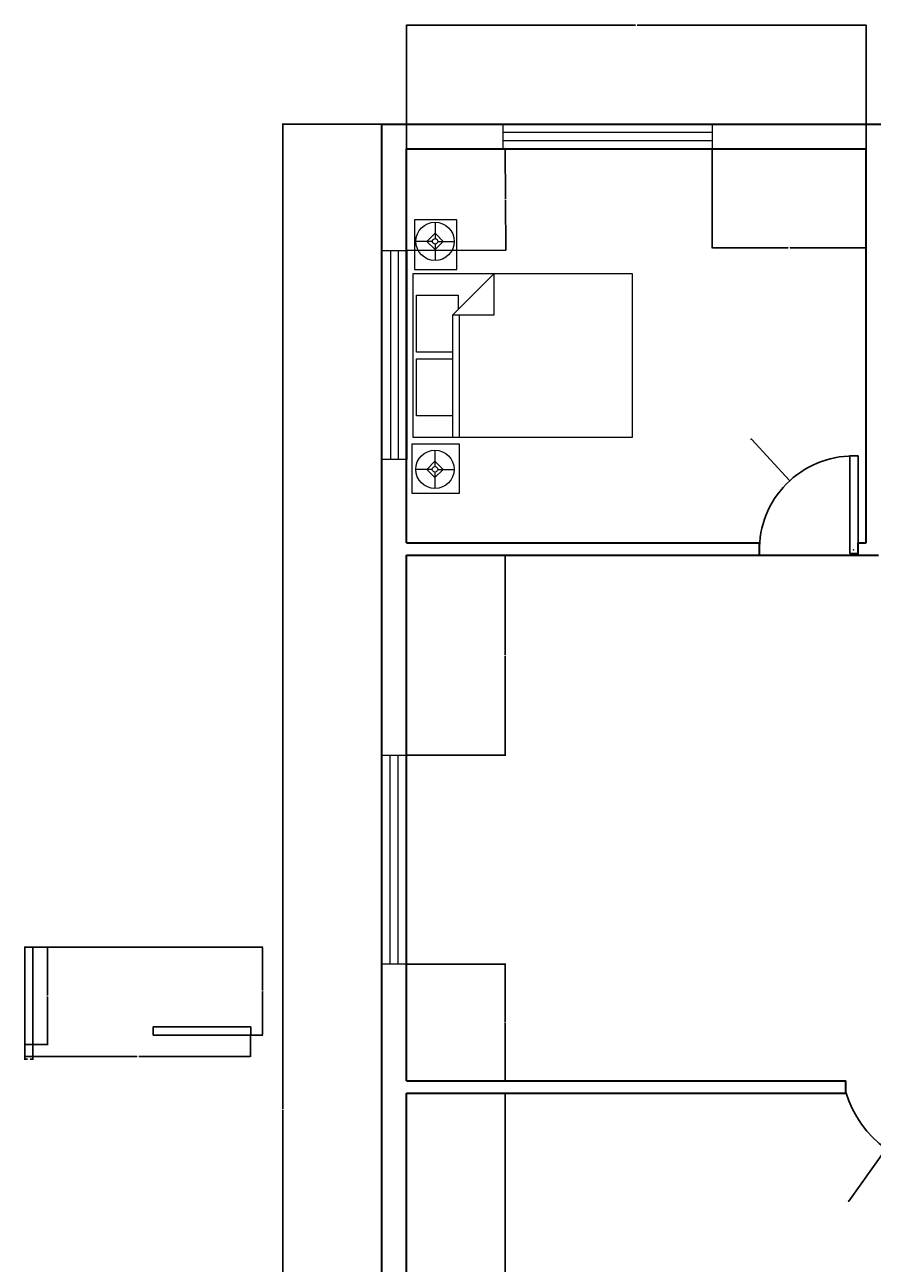
# Model space of a CAD drawing. Units: inches. Extents: x -52 to 1967, y 32 to 824.
# Tile 2 of 10: x 93 to 402, y 372 to 824. Entities that reach past the tile are written whole.
import ezdxf

# ---------------------------------------------------------------- set-up
doc = ezdxf.new("R2010")
doc.units = ezdxf.units.IN
for name, color, linetype, lineweight in [('A-ANNO-DIMS', 2, 'Continuous', 18), ('A-DOOR', 3, 'Continuous', 25), ('A-FURN', 8, 'Continuous', 18), ('A-GLAZ', 4, 'Continuous', 18), ('A-WALL', 7, 'Continuous', 35)]:
    doc.layers.add(name, color=color, linetype=linetype, lineweight=lineweight)
doc.styles.get("Standard").update_dxf_attribs({"font": 'arial.ttf'})
doc.dimstyles.get("Standard").update_dxf_attribs({"dimtxt": 0.18, "dimasz": 0.18, "dimexe": 0.18, "dimexo": 0.0625, "dimgap": 0.09, "dimtad": 0, "dimtih": 1, "dimtoh": 1, "dimdec": 4, "dimzin": 0, "dimdsep": 46, "dimtxsty": 'Standard', "dimcen": 0.09, "dimadec": 0, "dimazin": 0, "dimtfac": 1, "dimtdec": 4, "dimtofl": 0, "dimtmove": 0, "dimatfit": 3, "dimfxl": 1, "dimtolj": 1, "dimtzin": 0, "dimarcsym": 0})

# ---------------------------------------------------------------- blocks, each defined once
blk = doc.blocks.new('WIN-WIDE-76IN')
for p, q in [((0, 0), (0, 9)), ((0, 9), (76.34, 9)), ((76.34, 6), (0, 6)), ((76.34, 9), (76.34, 0)), ((0, 3), (76.34, 3)), ((76.34, 0), (0, 0))]:
    blk.add_line(p, q)
blk = doc.blocks.new('DOOR-LEAF-36IN')
blk.add_lwpolyline([(0, 0), (-2.98, 0), (-2.98, 35.63), (0, 35.63)], close=True)
blk = doc.blocks.new('Bed - Queen')
for p, q in [((0, -80.00003), (0, 0)), ((0, 0), (59.99999, 0)), ((59.99999, 0), (59.99999, -80.00003)), ((7.99999, -1.2), (28.79998, -1.2)), ((7.99999, -14.4), (7.99999, -1.2)), ((28.79998, -1.2), (28.79998, -14.4)), ((31.19999, -1.2), (51.99999, -1.2)), ((31.19999, -14.4), (31.19999, -1.2)), ((51.99999, -1.2), (51.99999, -16.4)), ((0, -14.4), (44.8, -14.4)), ((44.8, -16.8), (0, -16.8)), ((59.99999, -29.6), (44.8, -14.4)), ((44.8, -14.4), (44.8, -29.6)), ((51.99999, -16.4), (46.79936, -16.4)), ((44.8, -29.6), (59.99999, -29.6)), ((59.99999, -80.00003), (0, -80.00003))]:
    blk.add_line(p, q)
blk = doc.blocks.new('Lamp - Table')
for p, q in [((0, 7), (0, 1)), ((-1, 0), (-7, 0)), ((0, 3), (-3, 0)), ((-3, 0), (0, -3)), ((3, 0), (0, 3)), ((0, -3), (3, 0)), ((1, 0), (7, 0)), ((0, -1), (0, -7))]:
    blk.add_line(p, q)
for radius in [7, 1]:
    blk.add_circle((0, 0), radius)
blk = doc.blocks.new('BED-QUEEN-WITH-NIGHTSTANDS')
for points in [[(0.4, 61.39), (15.92, 61.39), (15.92, 79.53), (0.4, 79.53)], [(-0.42, -2.26), (16.73, -2.26), (16.73, -20.45), (-0.42, -20.45)]]:
    blk.add_lwpolyline(points, close=True)
for p in [(7.97, 71.69), (7.93, -11.61)]:
    blk.add_blockref('Lamp - Table', p)
at = {"rotation": 90}
blk.add_blockref('Bed - Queen', (0, 0), dxfattribs=at)
blk = doc.blocks.new('*D25')
at = {"layer": 'A-ANNO-DIMS', "color": 0, "lineweight": -2, "transparency": 16777216}
for p, q in [((95.68, 487.31), (101.14, 487.31)), ((100.96, 487.13), (100.96, 469.68)), ((100.96, 451.86), (100.96, 469.31)), ((95.68, 451.68), (101.14, 451.68))]:
    blk.add_line(p, q, dxfattribs=at)
at = {"layer": 'A-ANNO-DIMS', "color": 0, "transparency": 16777216}
for points in [[(100.93, 487.13), (100.99, 487.13), (100.96, 487.31)], [(100.93, 451.86), (100.99, 451.86), (100.96, 451.68)]]:
    blk.add_solid(points, dxfattribs=at)
at = {"layer": 'Defpoints', "color": 0, "transparency": 16777216}
for p in [(95.62, 487.31), (100.96, 487.31), (95.62, 451.68)]:
    blk.add_point(p, dxfattribs=at)
at = {"layer": 'A-ANNO-DIMS', "color": 0, "transparency": 16777216, "insert": (100.96, 469.49), "char_height": 0.18, "attachment_point": 5}
blk.add_mtext('\\A1;LEAF 36 TYP.', dxfattribs=at)
blk = doc.blocks.new('*D26')
at = {"layer": 'A-ANNO-DIMS', "color": 0, "lineweight": -2, "transparency": 16777216}
for p, q in [((92.64, 451.62), (92.64, 446.16)), ((95.62, 451.62), (95.62, 446.16)), ((92.82, 446.34), (93.67, 446.34)), ((95.44, 446.34), (94.59, 446.34))]:
    blk.add_line(p, q, dxfattribs=at)
at = {"layer": 'A-ANNO-DIMS', "color": 0, "transparency": 16777216}
for points in [[(92.82, 446.37), (92.82, 446.31), (92.64, 446.34)], [(95.44, 446.37), (95.44, 446.31), (95.62, 446.34)]]:
    blk.add_solid(points, dxfattribs=at)
at = {"layer": 'Defpoints', "color": 0, "transparency": 16777216}
for p in [(92.64, 451.68), (95.62, 451.68), (95.62, 446.34)]:
    blk.add_point(p, dxfattribs=at)
at = {"layer": 'A-ANNO-DIMS', "color": 0, "transparency": 16777216, "insert": (94.13, 446.34), "char_height": 0.18, "attachment_point": 5}
blk.add_mtext('\\A1;3 TYP.', dxfattribs=at)
blk = doc.blocks.new('*D54')
at = {"layer": 'A-ANNO-DIMS', "color": 0, "lineweight": -2, "transparency": 16777216}
for p, q in [((222.96, 787.97), (186.72, 787.97)), ((186.9, 787.79), (186.9, 428.16)), ((186.9, 68.15), (186.9, 427.79)), ((222.96, 67.97), (186.72, 67.97))]:
    blk.add_line(p, q, dxfattribs=at)
at = {"layer": 'A-ANNO-DIMS', "color": 0, "transparency": 16777216}
for points in [[(186.87, 787.79), (186.93, 787.79), (186.9, 787.97)], [(186.87, 68.15), (186.93, 68.15), (186.9, 67.97)]]:
    blk.add_solid(points, dxfattribs=at)
at = {"layer": 'Defpoints', "color": 0, "transparency": 16777216}
for p in [(186.9, 787.97), (223.03, 787.97), (223.03, 67.97)]:
    blk.add_point(p, dxfattribs=at)
at = {"layer": 'A-ANNO-DIMS', "color": 0, "transparency": 16777216, "insert": (186.9, 427.97), "char_height": 0.18, "attachment_point": 5}
blk.add_mtext('\\A1;720', dxfattribs=at)
blk = doc.blocks.new('*D55')
at = {"layer": 'A-ANNO-DIMS', "color": 0, "lineweight": -2, "transparency": 16777216}
for p, q in [((232.03, 779.04), (232.03, 824.32)), ((232.21, 824.14), (315.75, 824.14)), ((399.85, 824.14), (316.31, 824.14)), ((400.03, 779.04), (400.03, 824.32))]:
    blk.add_line(p, q, dxfattribs=at)
at = {"layer": 'A-ANNO-DIMS', "color": 0, "transparency": 16777216}
for points in [[(232.21, 824.17), (232.21, 824.11), (232.03, 824.14)], [(399.85, 824.17), (399.85, 824.11), (400.03, 824.14)]]:
    blk.add_solid(points, dxfattribs=at)
at = {"layer": 'Defpoints', "color": 0, "transparency": 16777216}
for p in [(400.03, 824.14), (232.03, 778.97), (400.03, 778.97)]:
    blk.add_point(p, dxfattribs=at)
at = {"layer": 'A-ANNO-DIMS', "color": 0, "transparency": 16777216, "insert": (316.03, 824.14), "char_height": 0.18, "attachment_point": 5}
blk.add_mtext('\\A1;168', dxfattribs=at)
blk = doc.blocks.new('*D59')
at = {"layer": 'A-ANNO-DIMS', "color": 0, "lineweight": -2, "transparency": 16777216}
for p, q in [((232.09, 630.47), (268.34, 630.47)), ((268.16, 630.29), (268.16, 594.14)), ((268.16, 557.62), (268.16, 593.77)), ((232.09, 557.44), (268.34, 557.44))]:
    blk.add_line(p, q, dxfattribs=at)
at = {"layer": 'A-ANNO-DIMS', "color": 0, "transparency": 16777216}
for points in [[(268.19, 630.29), (268.13, 630.29), (268.16, 630.47)], [(268.19, 557.62), (268.13, 557.62), (268.16, 557.44)]]:
    blk.add_solid(points, dxfattribs=at)
at = {"layer": 'Defpoints', "color": 0, "transparency": 16777216}
for p in [(232.03, 630.47), (232.03, 557.44), (268.16, 557.44)]:
    blk.add_point(p, dxfattribs=at)
at = {"layer": 'A-ANNO-DIMS', "color": 0, "transparency": 16777216, "insert": (268.16, 593.96), "char_height": 0.18, "attachment_point": 5}
blk.add_mtext('\\A1;73.03', dxfattribs=at)
blk = doc.blocks.new('*D60')
at = {"layer": 'A-ANNO-DIMS', "color": 0, "lineweight": -2, "transparency": 16777216}
for p, q in [((232.09, 433.97), (268.34, 433.97)), ((268.16, 433.79), (268.16, 356.16)), ((268.16, 278.15), (268.16, 355.79)), ((232.09, 277.97), (268.34, 277.97))]:
    blk.add_line(p, q, dxfattribs=at)
at = {"layer": 'A-ANNO-DIMS', "color": 0, "transparency": 16777216}
for points in [[(268.13, 433.79), (268.19, 433.79), (268.16, 433.97)], [(268.13, 278.15), (268.19, 278.15), (268.16, 277.97)]]:
    blk.add_solid(points, dxfattribs=at)
at = {"layer": 'Defpoints', "color": 0, "transparency": 16777216}
for p in [(232.03, 433.97), (232.03, 277.97), (268.16, 277.97)]:
    blk.add_point(p, dxfattribs=at)
at = {"layer": 'A-ANNO-DIMS', "color": 0, "transparency": 16777216, "insert": (268.16, 355.97), "char_height": 0.18, "attachment_point": 5}
blk.add_mtext('\\A1;156', dxfattribs=at)
blk = doc.blocks.new('*D75')
at = {"layer": 'A-ANNO-DIMS', "color": 0, "lineweight": -2, "transparency": 16777216}
for p, q in [((343.71, 778.92), (343.7, 742.68)), ((400.03, 778.91), (400.02, 742.66)), ((343.88, 742.86), (371.46, 742.85)), ((399.84, 742.84), (372.25, 742.85))]:
    blk.add_line(p, q, dxfattribs=at)
at = {"layer": 'A-ANNO-DIMS', "color": 0, "transparency": 16777216}
for points in [[(343.88, 742.89), (343.88, 742.83), (343.7, 742.86)], [(399.84, 742.87), (399.84, 742.81), (400.02, 742.84)]]:
    blk.add_solid(points, dxfattribs=at)
at = {"layer": 'Defpoints', "color": 0, "transparency": 16777216}
for p in [(343.71, 778.99), (400.03, 778.97), (343.7, 742.86)]:
    blk.add_point(p, dxfattribs=at)
at = {"layer": 'A-ANNO-DIMS', "color": 0, "transparency": 16777216, "insert": (371.86, 742.85), "char_height": 0.18, "attachment_point": 5}
blk.add_mtext('\\A1;56.32', dxfattribs=at)
blk = doc.blocks.new('*D87')
at = {"layer": 'A-ANNO-DIMS', "color": 0, "lineweight": -2, "transparency": 16777216}
for p, q in [((232.09, 778.97), (268.34, 779.13)), ((268.16, 778.95), (268.24, 760.72)), ((268.32, 742.13), (268.24, 760.35)), ((232.25, 741.79), (268.5, 741.95))]:
    blk.add_line(p, q, dxfattribs=at)
at = {"layer": 'A-ANNO-DIMS', "color": 0, "transparency": 16777216}
for points in [[(268.19, 778.95), (268.13, 778.95), (268.16, 779.13)], [(268.35, 742.13), (268.29, 742.12), (268.32, 741.95)]]:
    blk.add_solid(points, dxfattribs=at)
at = {"layer": 'Defpoints', "color": 0, "transparency": 16777216}
for p in [(232.03, 778.97), (232.19, 741.79), (268.32, 741.95)]:
    blk.add_point(p, dxfattribs=at)
at = {"layer": 'A-ANNO-DIMS', "color": 0, "transparency": 16777216, "insert": (268.24, 760.54), "char_height": 0.18, "attachment_point": 5}
blk.add_mtext('\\A1;37.184', dxfattribs=at)
blk = doc.blocks.new('*D88')
at = {"layer": 'A-ANNO-DIMS', "color": 0, "lineweight": -2, "transparency": 16777216}
for p, q in [((232.09, 481.1), (268.34, 481.1)), ((268.16, 480.92), (268.16, 459.97)), ((268.16, 438.65), (268.16, 459.6)), ((232.09, 438.47), (268.34, 438.47))]:
    blk.add_line(p, q, dxfattribs=at)
at = {"layer": 'A-ANNO-DIMS', "color": 0, "transparency": 16777216}
for points in [[(268.13, 480.92), (268.19, 480.92), (268.16, 481.1)], [(268.13, 438.65), (268.19, 438.65), (268.16, 438.47)]]:
    blk.add_solid(points, dxfattribs=at)
at = {"layer": 'Defpoints', "color": 0, "transparency": 16777216}
for p in [(232.03, 481.1), (232.03, 438.47), (268.16, 438.47)]:
    blk.add_point(p, dxfattribs=at)
at = {"layer": 'A-ANNO-DIMS', "color": 0, "transparency": 16777216, "insert": (268.16, 459.79), "char_height": 0.18, "attachment_point": 5}
blk.add_mtext('\\A1;42.625', dxfattribs=at)
blk = doc.blocks.new('*D122')
at = {"layer": 'A-ANNO-DIMS', "color": 0, "lineweight": -2, "transparency": 16777216}
for p, q in [((175.15, 455.1), (175.15, 447.2)), ((92.64, 451.62), (92.64, 447.2)), ((92.82, 447.38), (133.52, 447.38)), ((174.97, 447.38), (134.27, 447.38))]:
    blk.add_line(p, q, dxfattribs=at)
at = {"layer": 'A-ANNO-DIMS', "color": 0, "transparency": 16777216}
for points in [[(92.82, 447.41), (92.82, 447.35), (92.64, 447.38)], [(174.97, 447.41), (174.97, 447.35), (175.15, 447.38)]]:
    blk.add_solid(points, dxfattribs=at)
at = {"layer": 'Defpoints', "color": 0, "transparency": 16777216}
for p in [(175.15, 455.16), (92.64, 451.68), (175.15, 447.38)]:
    blk.add_point(p, dxfattribs=at)
at = {"layer": 'A-ANNO-DIMS', "color": 0, "transparency": 16777216, "insert": (133.89, 447.38), "char_height": 0.18, "attachment_point": 5}
blk.add_mtext('\\A1;82.51', dxfattribs=at)
blk = doc.blocks.new('*D123')
at = {"layer": 'A-ANNO-DIMS', "color": 0, "lineweight": -2, "transparency": 16777216}
for p, q in [((95.68, 487.31), (179.63, 487.31)), ((179.45, 487.13), (179.45, 471.42)), ((179.45, 455.34), (179.45, 471.05)), ((139.59, 455.16), (179.63, 455.16))]:
    blk.add_line(p, q, dxfattribs=at)
at = {"layer": 'A-ANNO-DIMS', "color": 0, "transparency": 16777216}
for points in [[(179.42, 487.13), (179.48, 487.13), (179.45, 487.31)], [(179.42, 455.34), (179.48, 455.34), (179.45, 455.16)]]:
    blk.add_solid(points, dxfattribs=at)
at = {"layer": 'Defpoints', "color": 0, "transparency": 16777216}
for p in [(95.62, 487.31), (139.52, 455.16), (179.45, 455.16)]:
    blk.add_point(p, dxfattribs=at)
at = {"layer": 'A-ANNO-DIMS', "color": 0, "transparency": 16777216, "insert": (179.45, 471.23), "char_height": 0.18, "attachment_point": 5}
blk.add_mtext('\\A1;32.146', dxfattribs=at)
blk = doc.blocks.new('*D135')
at = {"layer": 'A-ANNO-DIMS', "color": 0, "lineweight": -2, "transparency": 16777216}
for p, q in [((430, 445.49), (430.18, 445.49)), ((430.09, 445.4), (430.09, 445.58)), ((393.63, 394.5), (407.2, 413.48)), ((393.45, 394.5), (393.63, 394.5))]:
    blk.add_line(p, q, dxfattribs=at)
at = {"layer": 'A-ANNO-DIMS', "color": 0, "transparency": 16777216}
blk.add_solid([(407.18, 413.49), (407.22, 413.46), (407.3, 413.62)], dxfattribs=at)
at = {"layer": 'Defpoints', "color": 0, "transparency": 16777216}
for p in [(430.09, 445.49), (407.3, 413.62)]:
    blk.add_point(p, dxfattribs=at)
at = {"layer": 'A-ANNO-DIMS', "color": 0, "transparency": 16777216, "insert": (392.97, 394.5), "char_height": 0.18, "attachment_point": 5}
blk.add_mtext('\\A1;R39.17', dxfattribs=at)
blk = doc.blocks.new('*D139')
at = {"layer": 'A-ANNO-DIMS', "color": 0, "lineweight": -2, "transparency": 16777216}
for p, q in [((357.92, 672.85), (358.1, 672.85)), ((358.1, 672.85), (371.94, 657.83)), ((395.24, 632.46), (395.42, 632.46)), ((395.33, 632.37), (395.33, 632.55))]:
    blk.add_line(p, q, dxfattribs=at)
at = {"layer": 'A-ANNO-DIMS', "color": 0, "transparency": 16777216}
blk.add_solid([(371.96, 657.85), (371.92, 657.81), (372.06, 657.7)], dxfattribs=at)
at = {"layer": 'Defpoints', "color": 0, "transparency": 16777216}
for p in [(372.06, 657.7), (395.33, 632.46)]:
    blk.add_point(p, dxfattribs=at)
at = {"layer": 'A-ANNO-DIMS', "color": 0, "transparency": 16777216, "insert": (357.44, 672.85), "char_height": 0.18, "attachment_point": 5}
blk.add_mtext('\\A1;R34.33', dxfattribs=at)

msp = doc.modelspace()

# ---------------------------------------------------------------- linework, layer by layer
at = {"layer": 'A-DOOR'}
for centre, radius, start, end in [((395.3328, 632.4601), 34.3327, 87.22099, 178.126829), ((430.0876, 445.4886), 39.1725, 196.688789, 272.182514)]:
    msp.add_arc(centre, radius, start, end, dxfattribs=at)
at = {"layer": 'A-WALL'}
for p, q in [((223.0273, 67.9731), (223.0273, 787.9731)), ((223.0273, 787.9731), (703.0273, 787.9731)), ((232.0273, 778.9731), (400.0273, 778.9731)), ((232.0273, 634.9731), (232.0273, 778.9731)), ((400.0273, 634.9731), (400.0273, 778.9731)), ((232.0273, 634.9731), (361.0273, 634.9731)), ((361.0273, 630.4731), (361.0273, 634.9731)), ((397.0273, 630.4731), (397.0273, 634.9731)), ((397.0273, 634.9731), (400.0273, 634.9731)), ((232.0273, 630.4731), (404.5273, 630.4731)), ((232.0273, 438.4731), (232.0273, 630.4731)), ((232.0273, 438.4731), (392.5273, 438.4731)), ((392.5273, 433.9731), (392.5273, 438.4731)), ((232.0273, 433.9731), (392.5273, 433.9731)), ((232.0273, 277.9731), (232.0273, 433.9731))]:
    msp.add_line(p, q, dxfattribs=at)

# ---------------------------------------------------------------- block references
at = {"layer": 'A-DOOR'}
for p in [(397.0194, 631.1402), (95.6204, 451.6803)]:
    msp.add_blockref('DOOR-LEAF-36IN', p, dxfattribs=at)
at = {"layer": 'A-DOOR', "rotation": 270.0000000000001}
msp.add_blockref('DOOR-LEAF-36IN', (139.523, 455.1602), dxfattribs=at)
at = {"layer": 'A-FURN'}
msp.add_blockref('BED-QUEEN-WITH-NIGHTSTANDS', (234.5515, 673.4827), dxfattribs=at)
at = {"layer": 'A-GLAZ'}
msp.add_blockref('WIN-WIDE-76IN', (267.3656, 778.987), dxfattribs=at)
for p, rotation in [((223.1875, 741.7894), 270), ((223.028, 557.4384), 270.0000000000001)]:
    msp.add_blockref('WIN-WIDE-76IN', p, dxfattribs=dict(at, rotation=rotation))

# ---------------------------------------------------------------- dimensions: what is measured, and where the dimension line sits
at = {"layer": 'A-ANNO-DIMS'}
for base, p1, p2, override, picture, middle in [((400.0273, 824.138), (232.0273, 778.9731), (400.0273, 778.9731), {"dimdec": 0, "dimlfac": 1, "dimrnd": 0, "dimzin": 0, "dimdsep": 46, "dimlunit": 2}, '*D55', (316.0273, 824.138)), ((175.1487, 447.3803), (92.636, 451.6803), (175.1487, 455.1602), {"dimdec": 2, "dimlfac": 1, "dimrnd": 0, "dimzin": 0, "dimdsep": 46, "dimlunit": 2}, '*D122', (133.8924, 447.3803))]:
    dim = msp.add_linear_dim(base=base, p1=p1, p2=p2, dimstyle='Standard', override=override, dxfattribs=at)
    dim.commit()
    dim.dimension.update_dxf_attribs({"geometry": picture, "text_midpoint": middle})
for base, p1, p2, angle, override, picture, middle in [((186.8973, 787.9731), (223.0273, 67.9731), (223.0273, 787.9731), 90, {"dimdec": 0, "dimlfac": 1, "dimrnd": 0, "dimzin": 0, "dimdsep": 46, "dimlunit": 2}, '*D54', (186.8973, 427.9731)), ((268.3171, 741.945), (232.0273, 778.9731), (232.1875, 741.7894), 270.246839, {"dimdec": 3, "dimlfac": 1, "dimrnd": 0, "dimzin": 0, "dimdsep": 46, "dimlunit": 2}, '*D87', (268.237, 760.5369)), ((343.6969, 742.857), (400.0273, 778.9731), (343.7057, 778.987), 179.985936, {"dimdec": 2, "dimlfac": 1, "dimrnd": 0, "dimzin": 0, "dimdsep": 46, "dimlunit": 2}, '*D75', (371.8576, 742.8501)), ((268.158, 557.4388), (232.0273, 630.4731), (232.028, 557.4384), 270.00061, {"dimdec": 2, "dimlfac": 1, "dimrnd": 0, "dimzin": 0, "dimdsep": 46, "dimlunit": 2}, '*D59', (268.1577, 593.9561)), ((179.4487, 455.1602), (95.6204, 487.306), (139.523, 455.1602), 90, {"dimdec": 3, "dimlfac": 1, "dimrnd": 0, "dimzin": 0, "dimdsep": 46, "dimlunit": 2}, '*D123', (179.4487, 471.2331)), ((268.1573, 438.4725), (232.028, 481.0982), (232.0273, 438.4731), 269.998956, {"dimdec": 3, "dimlfac": 1, "dimrnd": 0, "dimzin": 0, "dimdsep": 46, "dimlunit": 2}, '*D88', (268.1577, 459.785)), ((268.1573, 277.9731), (232.0273, 433.9731), (232.0273, 277.9731), 270, {"dimdec": 0, "dimlfac": 1, "dimrnd": 0, "dimzin": 0, "dimdsep": 46, "dimlunit": 2}, '*D60', (268.1573, 355.9731))]:
    dim = msp.add_linear_dim(base=base, p1=p1, p2=p2, angle=angle, dimstyle='Standard', override=override, dxfattribs=at)
    dim.commit()
    dim.dimension.update_dxf_attribs({"geometry": picture, "text_midpoint": middle})
for center, mpoint, picture, middle in [((395.3328, 632.4601), (372.061, 657.702), '*D139', (357.438, 672.8472)), ((430.0876, 445.4886), (407.3042, 413.6232), '*D135', (392.9743, 394.504))]:
    dim = msp.add_radius_dim(center=center, mpoint=mpoint, dimstyle='Standard', override={"dimdec": 2, "dimlfac": 1, "dimrnd": 0, "dimzin": 0, "dimdsep": 46, "dimlunit": 2}, dxfattribs=at)
    dim.commit()
    dim.dimension.update_dxf_attribs({"geometry": picture, "text_midpoint": middle, "dimtype": 164})
dim = msp.add_linear_dim(base=(100.9642, 487.306), p1=(95.6204, 451.6803), p2=(95.6204, 487.306), angle=90, text='LEAF <> TYP.', dimstyle='Standard', override={"dimdec": 0, "dimlfac": 1, "dimrnd": 0, "dimzin": 0, "dimdsep": 46, "dimlunit": 2}, dxfattribs=at)
dim.commit()
dim.dimension.update_dxf_attribs({"geometry": '*D25', "text_midpoint": (100.9642, 469.4931)})
dim = msp.add_linear_dim(base=(95.6204, 446.3364), p1=(92.636, 451.6803), p2=(95.6204, 451.6803), text='<> TYP.', dimstyle='Standard', override={"dimdec": 0, "dimlfac": 1, "dimrnd": 0, "dimzin": 0, "dimdsep": 46, "dimlunit": 2}, dxfattribs=at)
dim.commit()
dim.dimension.update_dxf_attribs({"geometry": '*D26', "text_midpoint": (94.1282, 446.3364)})

doc.saveas('drawing.dxf')
